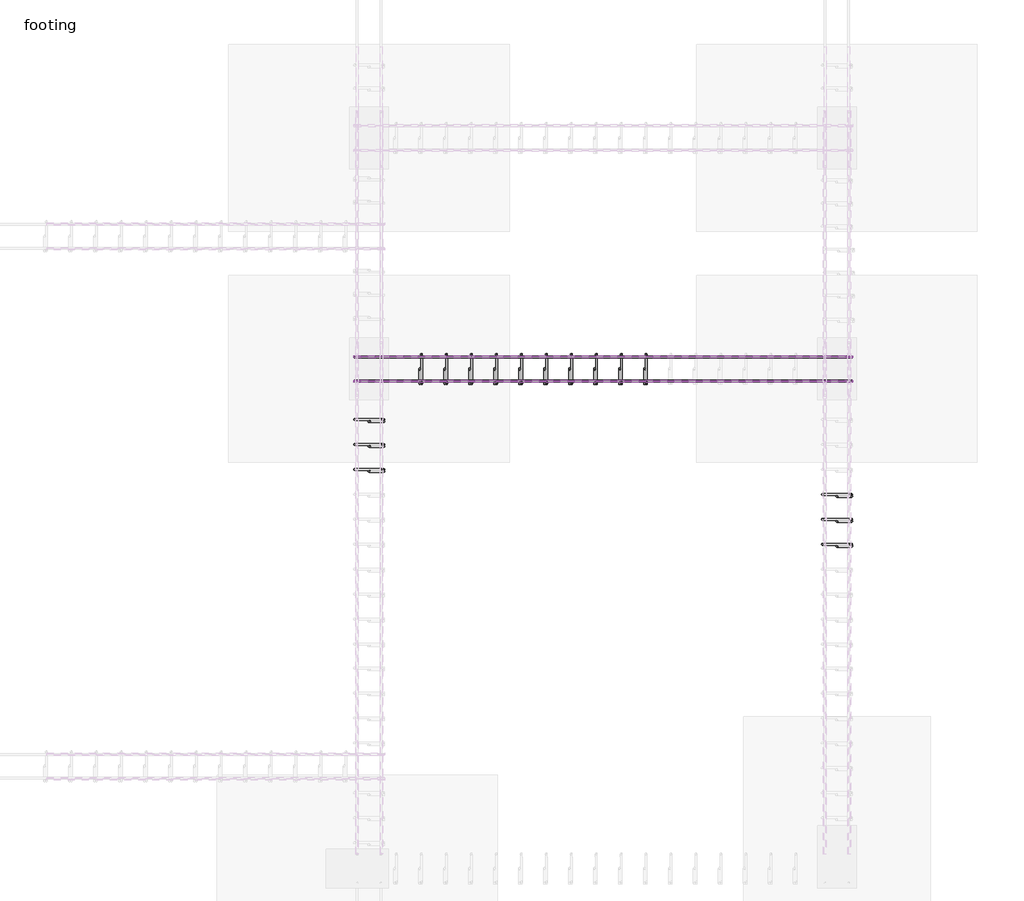
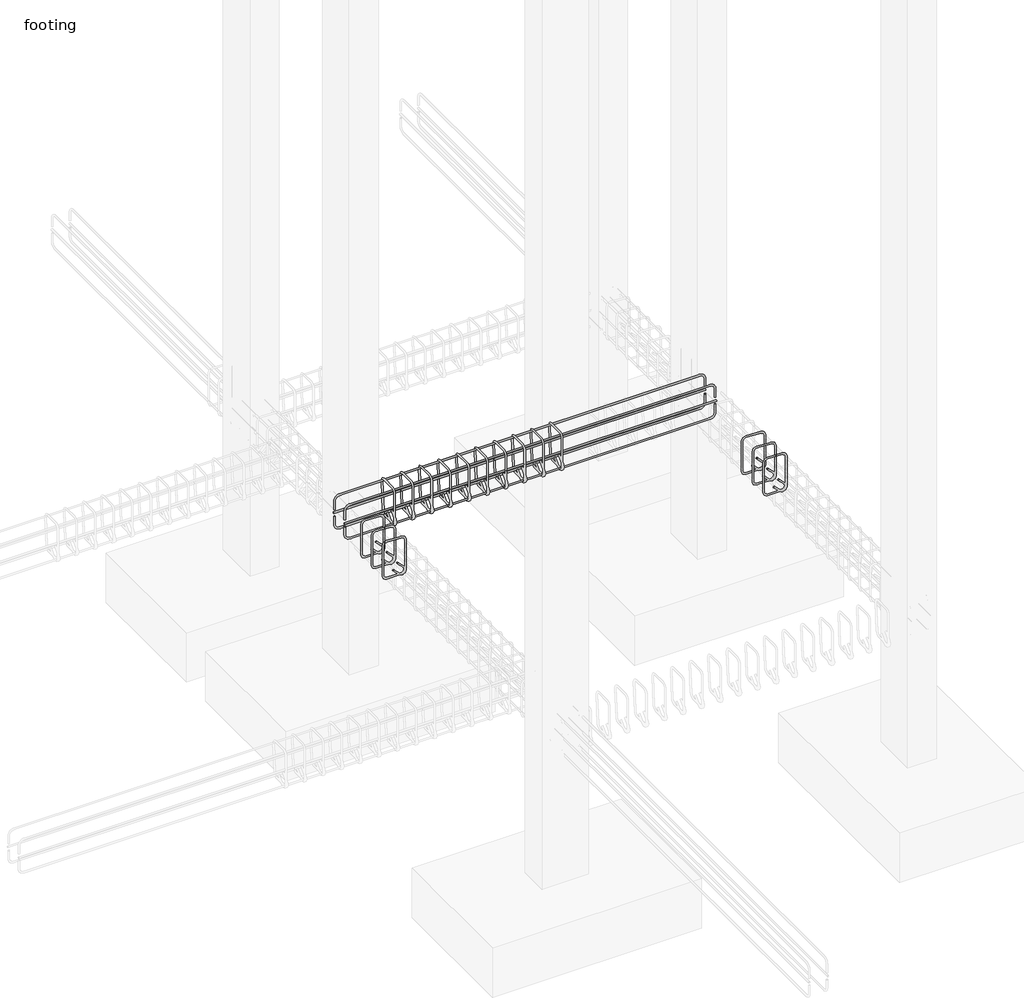
# One storey, part 13 of 21: 22 reinforcing bars.
"""IFC4 building model written with IfcOpenShell, lengths in millimetres."""

from ifc_helpers import new_model, si_unit, point, frame, origin, place, context, project, spatial, polyline, circle_curve, trimmed, segment, composite_curve, element, save
from ifc_brep_helpers import swept_disk

model = new_model("IFC4")

# Units and contexts
model_context = context("Model", 3, world=origin())
ifc_project = project(units=[si_unit("LENGTHUNIT", "METRE", prefix="MILLI")], contexts=[model_context])

# Site, building, storey
site = spatial("IfcSite", under=ifc_project)
building = spatial("IfcBuilding", under=site)
storey = spatial("IfcBuildingStorey", under=building, Name="footing", Elevation=-1524.0)

# Reinforcing bars
placement = place(None, origin())
element("IfcReinforcingBar", 1, at=placement, inside=storey, context=model_context, shape_type="SolidModel", body=[
    swept_disk(composite_curve([segment(polyline([(-4722.5521673, 6772.6372086, -236.1172592), (-4722.5521673, 6772.6372086, -312.3172592)]), True, "CONTINUOUS"), segment(trimmed(circle_curve(frame((-4767.0021673, 6772.6372086, -312.3172592), z_axis=(0.0, 1.0, -2.1166279873208456e-12), x_axis=(44.44999999999982, 0.0, 0.0)), 44.45), [point((-4722.5521673, 6772.6372086, -312.3172592))], [point((-4767.0021673, 6772.6372086, -356.7672592))], True, "CARTESIAN"), True, "CONTINUOUS"), segment(polyline([(-4767.0021673, 6772.6372086, -356.7672592), (-7917.3959173, 6772.6372086, -356.7672592)]), True, "CONTINUOUS"), segment(trimmed(circle_curve(frame((-7917.3959173, 6772.6372086, -312.3172592), z_axis=(0.0, 1.0, -2.1166279873208456e-12), x_axis=(0.0, 0.0, -44.44999999999999)), 44.45), [point((-7917.3959173, 6772.6372086, -356.7672592))], [point((-7961.8459173, 6772.6372086, -312.3172592))], True, "CARTESIAN"), True, "CONTINUOUS"), segment(polyline([(-7961.8459173, 6772.6372086, -312.3172592), (-7961.8459173, 6772.6372086, -236.1172592)]), True, "CONTINUOUS")], self_intersect=False), 6.35),
])
element("IfcReinforcingBar", 2, at=placement, inside=storey, context=model_context, shape_type="SolidModel", body=[
    swept_disk(composite_curve([segment(polyline([(-4722.5521673, 6617.9026902, -170.2827408), (-4722.5521673, 6617.9026902, -94.0827408)]), True, "CONTINUOUS"), segment(trimmed(circle_curve(frame((-4767.0021673, 6617.9026902, -94.0827408), z_axis=(0.0, -1.0, 0.0), x_axis=(44.44999999999982, 0.0, 0.0)), 44.45), [point((-4722.5521673, 6617.9026902, -94.0827408))], [point((-4767.0021673, 6617.9026902, -49.6327408))], True, "CARTESIAN"), True, "CONTINUOUS"), segment(polyline([(-4767.0021673, 6617.9026902, -49.6327408), (-7917.3959173, 6617.9026902, -49.6327408)]), True, "CONTINUOUS"), segment(trimmed(circle_curve(frame((-7917.3959173, 6617.9026902, -94.0827408), z_axis=(0.0, -1.0, 0.0), x_axis=(0.0, 0.0, 44.449999999999996)), 44.45), [point((-7917.3959173, 6617.9026902, -49.6327408))], [point((-7961.8459173, 6617.9026902, -94.0827408))], True, "CARTESIAN"), True, "CONTINUOUS"), segment(polyline([(-7961.8459173, 6617.9026902, -94.0827408), (-7961.8459173, 6617.9026902, -170.2827408)]), True, "CONTINUOUS")], self_intersect=False), 6.35),
])
element("IfcReinforcingBar", 3, at=placement, inside=storey, context=model_context, shape_type="SolidModel", body=[
    swept_disk(composite_curve([segment(polyline([(-4722.5521673, 6617.9026902, -236.1172592), (-4722.5521673, 6617.9026902, -312.3172592)]), True, "CONTINUOUS"), segment(trimmed(circle_curve(frame((-4767.0021673, 6617.9026902, -312.3172592), z_axis=(0.0, 1.0, 2.1166279873208456e-12), x_axis=(44.44999999999982, 0.0, 0.0)), 44.45), [point((-4722.5521673, 6617.9026902, -312.3172592))], [point((-4767.0021673, 6617.9026902, -356.7672592))], True, "CARTESIAN"), True, "CONTINUOUS"), segment(polyline([(-4767.0021673, 6617.9026902, -356.7672592), (-7917.3959173, 6617.9026902, -356.7672592)]), True, "CONTINUOUS"), segment(trimmed(circle_curve(frame((-7917.3959173, 6617.9026902, -312.3172592), z_axis=(0.0, 1.0, 2.1166279873208456e-12), x_axis=(0.0, 0.0, -44.44999999999999)), 44.45), [point((-7917.3959173, 6617.9026902, -356.7672592))], [point((-7961.8459173, 6617.9026902, -312.3172592))], True, "CARTESIAN"), True, "CONTINUOUS"), segment(polyline([(-7961.8459173, 6617.9026902, -312.3172592), (-7961.8459173, 6617.9026902, -236.1172592)]), True, "CONTINUOUS")], self_intersect=False), 6.35),
])
element("IfcReinforcingBar", 4, at=placement, inside=storey, context=model_context, shape_type="SolidModel", body=[
    swept_disk(composite_curve([segment(polyline([(-4722.5521673, 6772.6372086, -170.2827408), (-4722.5521673, 6772.6372086, -94.0827408)]), True, "CONTINUOUS"), segment(trimmed(circle_curve(frame((-4767.0021673, 6772.6372086, -94.0827408), z_axis=(0.0, -1.0, 0.0), x_axis=(44.44999999999982, 0.0, 0.0)), 44.45), [point((-4722.5521673, 6772.6372086, -94.0827408))], [point((-4767.0021673, 6772.6372086, -49.6327408))], True, "CARTESIAN"), True, "CONTINUOUS"), segment(polyline([(-4767.0021673, 6772.6372086, -49.6327408), (-7917.3959173, 6772.6372086, -49.6327408)]), True, "CONTINUOUS"), segment(trimmed(circle_curve(frame((-7917.3959173, 6772.6372086, -94.0827408), z_axis=(0.0, -1.0, 0.0), x_axis=(0.0, 0.0, 44.449999999999996)), 44.45), [point((-7917.3959173, 6772.6372086, -49.6327408))], [point((-7961.8459173, 6772.6372086, -94.0827408))], True, "CARTESIAN"), True, "CONTINUOUS"), segment(polyline([(-7961.8459173, 6772.6372086, -94.0827408), (-7961.8459173, 6772.6372086, -170.2827408)]), True, "CONTINUOUS")], self_intersect=False), 6.35),
])
element("IfcReinforcingBar", 5, at=placement, inside=storey, context=model_context, shape_type="SolidModel", body=[
    swept_disk(composite_curve([segment(polyline([(-4716.2021673, 6778.2168244, -203.2), (-7968.1959173, 6778.2168244, -203.2)]), True, "CONTINUOUS")], self_intersect=False), 6.35),
])
element("IfcReinforcingBar", 6, at=placement, inside=storey, context=model_context, shape_type="SolidModel", body=[
    swept_disk(composite_curve([segment(polyline([(-4716.2021673, 6612.3230744, -203.2), (-7968.1959173, 6612.3230744, -203.2)]), True, "CONTINUOUS")], self_intersect=False), 6.35),
])
element("IfcReinforcingBar", 7, at=placement, inside=storey, context=model_context, shape_type="SolidModel", body=[
    swept_disk(composite_curve([segment(polyline([(-7537.0883428, 6708.6887132, -310.8825168), (-7537.0883428, 6653.8237147, -365.7475153)]), True, "CONTINUOUS"), segment(trimmed(circle_curve(frame((-7537.0883428, 6631.3730744, -343.296875), z_axis=(-1.0, 0.0, 0.0), x_axis=(0.0, 22.450640299999577, -22.450640299999975)), 31.75), [point((-7537.0883428, 6653.8237147, -365.7475153))], [point((-7537.0883428, 6599.6230744, -343.296875))], True, "CARTESIAN"), True, "CONTINUOUS"), segment(polyline([(-7537.0883428, 6599.6230744, -343.296875), (-7537.0883428, 6599.6230744, -63.103125)]), True, "CONTINUOUS"), segment(trimmed(circle_curve(frame((-7537.0883428, 6631.3730744, -63.103125), z_axis=(-1.0, 0.0, 0.0), x_axis=(0.0, -31.75, 0.0)), 31.75), [point((-7537.0883428, 6599.6230744, -63.103125))], [point((-7537.0883428, 6631.3730744, -31.353125))], True, "CARTESIAN"), True, "CONTINUOUS"), segment(polyline([(-7537.0883428, 6631.3730744, -31.353125), (-7537.0883428, 6759.1668244, -31.353125)]), True, "CONTINUOUS"), segment(trimmed(circle_curve(frame((-7535.9159328, 6759.1668244, -63.0814712), z_axis=(-0.9993179916193466, 0.0, -0.03692629992126919), x_axis=(-1.1724100000001272, 0.0, 31.728346200000004)), 31.75), [point((-7537.0883428, 6759.1668244, -31.353125))], [point((-7535.9159328, 6790.9168244, -63.0814712))], True, "CARTESIAN"), True, "CONTINUOUS"), segment(polyline([(-7535.9159328, 6790.9168244, -63.0814712), (-7525.5607528, 6790.9168244, -343.3185288)]), True, "CONTINUOUS"), segment(trimmed(circle_curve(frame((-7525.5607528, 6759.1668244, -343.3185288), z_axis=(-0.9993179916193466, 0.0, -0.03692629992126919), x_axis=(0.0, 31.75, 0.0)), 31.75), [point((-7525.5607528, 6790.9168244, -343.3185288))], [point((-7524.3883428, 6759.1668244, -375.046875))], True, "CARTESIAN"), True, "CONTINUOUS"), segment(polyline([(-7524.3883428, 6759.1668244, -375.046875), (-7524.3883428, 6631.3730744, -375.046875)]), True, "CONTINUOUS"), segment(trimmed(circle_curve(frame((-7524.3883428, 6631.3730744, -343.296875), z_axis=(-1.0, 0.0, 0.0), x_axis=(0.0, 0.0, -31.75)), 31.75), [point((-7524.3883428, 6631.3730744, -375.046875))], [point((-7524.3883428, 6608.9224341, -320.8462347))], True, "CARTESIAN"), True, "CONTINUOUS"), segment(polyline([(-7524.3883428, 6608.9224341, -320.8462347), (-7524.3883428, 6663.7874326, -265.9812362)]), True, "CONTINUOUS")], self_intersect=False), 6.35),
])
element("IfcReinforcingBar", 8, at=placement, inside=storey, context=model_context, shape_type="SolidModel", body=[
    swept_disk(composite_curve([segment(polyline([(-7374.3883428, 6708.6887132, -310.8825168), (-7374.3883428, 6653.8237147, -365.7475153)]), True, "CONTINUOUS"), segment(trimmed(circle_curve(frame((-7374.3883428, 6631.3730744, -343.296875), z_axis=(-1.0, 0.0, 0.0), x_axis=(0.0, 22.450640299999577, -22.450640299999975)), 31.75), [point((-7374.3883428, 6653.8237147, -365.7475153))], [point((-7374.3883428, 6599.6230744, -343.296875))], True, "CARTESIAN"), True, "CONTINUOUS"), segment(polyline([(-7374.3883428, 6599.6230744, -343.296875), (-7374.3883428, 6599.6230744, -63.103125)]), True, "CONTINUOUS"), segment(trimmed(circle_curve(frame((-7374.3883428, 6631.3730744, -63.103125), z_axis=(-1.0, 0.0, 0.0), x_axis=(0.0, -31.75, 0.0)), 31.75), [point((-7374.3883428, 6599.6230744, -63.103125))], [point((-7374.3883428, 6631.3730744, -31.353125))], True, "CARTESIAN"), True, "CONTINUOUS"), segment(polyline([(-7374.3883428, 6631.3730744, -31.353125), (-7374.3883428, 6759.1668244, -31.353125)]), True, "CONTINUOUS"), segment(trimmed(circle_curve(frame((-7373.2159328, 6759.1668244, -63.0814712), z_axis=(-0.9993179916193466, 0.0, -0.03692629992126919), x_axis=(-1.1724100000001272, 0.0, 31.728346200000004)), 31.75), [point((-7374.3883428, 6759.1668244, -31.353125))], [point((-7373.2159328, 6790.9168244, -63.0814712))], True, "CARTESIAN"), True, "CONTINUOUS"), segment(polyline([(-7373.2159328, 6790.9168244, -63.0814712), (-7362.8607528, 6790.9168244, -343.3185288)]), True, "CONTINUOUS"), segment(trimmed(circle_curve(frame((-7362.8607528, 6759.1668244, -343.3185288), z_axis=(-0.9993179916193466, 0.0, -0.03692629992126919), x_axis=(0.0, 31.75, 0.0)), 31.75), [point((-7362.8607528, 6790.9168244, -343.3185288))], [point((-7361.6883428, 6759.1668244, -375.046875))], True, "CARTESIAN"), True, "CONTINUOUS"), segment(polyline([(-7361.6883428, 6759.1668244, -375.046875), (-7361.6883428, 6631.3730744, -375.046875)]), True, "CONTINUOUS"), segment(trimmed(circle_curve(frame((-7361.6883428, 6631.3730744, -343.296875), z_axis=(-1.0, 0.0, 0.0), x_axis=(0.0, 0.0, -31.75)), 31.75), [point((-7361.6883428, 6631.3730744, -375.046875))], [point((-7361.6883428, 6608.9224341, -320.8462347))], True, "CARTESIAN"), True, "CONTINUOUS"), segment(polyline([(-7361.6883428, 6608.9224341, -320.8462347), (-7361.6883428, 6663.7874326, -265.9812362)]), True, "CONTINUOUS")], self_intersect=False), 6.35),
])
element("IfcReinforcingBar", 9, at=placement, inside=storey, context=model_context, shape_type="SolidModel", body=[
    swept_disk(composite_curve([segment(polyline([(-7211.6883428, 6708.6887132, -310.8825168), (-7211.6883428, 6653.8237147, -365.7475153)]), True, "CONTINUOUS"), segment(trimmed(circle_curve(frame((-7211.6883428, 6631.3730744, -343.296875), z_axis=(-1.0, 0.0, 0.0), x_axis=(0.0, 22.450640299999577, -22.450640299999975)), 31.75), [point((-7211.6883428, 6653.8237147, -365.7475153))], [point((-7211.6883428, 6599.6230744, -343.296875))], True, "CARTESIAN"), True, "CONTINUOUS"), segment(polyline([(-7211.6883428, 6599.6230744, -343.296875), (-7211.6883428, 6599.6230744, -63.103125)]), True, "CONTINUOUS"), segment(trimmed(circle_curve(frame((-7211.6883428, 6631.3730744, -63.103125), z_axis=(-1.0, 0.0, 0.0), x_axis=(0.0, -31.75, 0.0)), 31.75), [point((-7211.6883428, 6599.6230744, -63.103125))], [point((-7211.6883428, 6631.3730744, -31.353125))], True, "CARTESIAN"), True, "CONTINUOUS"), segment(polyline([(-7211.6883428, 6631.3730744, -31.353125), (-7211.6883428, 6759.1668244, -31.353125)]), True, "CONTINUOUS"), segment(trimmed(circle_curve(frame((-7210.5159328, 6759.1668244, -63.0814712), z_axis=(-0.9993179916193466, 0.0, -0.03692629992126919), x_axis=(-1.1724100000001272, 0.0, 31.728346200000004)), 31.75), [point((-7211.6883428, 6759.1668244, -31.353125))], [point((-7210.5159328, 6790.9168244, -63.0814712))], True, "CARTESIAN"), True, "CONTINUOUS"), segment(polyline([(-7210.5159328, 6790.9168244, -63.0814712), (-7200.1607528, 6790.9168244, -343.3185288)]), True, "CONTINUOUS"), segment(trimmed(circle_curve(frame((-7200.1607528, 6759.1668244, -343.3185288), z_axis=(-0.9993179916193466, 0.0, -0.03692629992126919), x_axis=(0.0, 31.75, 0.0)), 31.75), [point((-7200.1607528, 6790.9168244, -343.3185288))], [point((-7198.9883428, 6759.1668244, -375.046875))], True, "CARTESIAN"), True, "CONTINUOUS"), segment(polyline([(-7198.9883428, 6759.1668244, -375.046875), (-7198.9883428, 6631.3730744, -375.046875)]), True, "CONTINUOUS"), segment(trimmed(circle_curve(frame((-7198.9883428, 6631.3730744, -343.296875), z_axis=(-1.0, 0.0, 0.0), x_axis=(0.0, 0.0, -31.75)), 31.75), [point((-7198.9883428, 6631.3730744, -375.046875))], [point((-7198.9883428, 6608.9224341, -320.8462347))], True, "CARTESIAN"), True, "CONTINUOUS"), segment(polyline([(-7198.9883428, 6608.9224341, -320.8462347), (-7198.9883428, 6663.7874326, -265.9812362)]), True, "CONTINUOUS")], self_intersect=False), 6.35),
])
element("IfcReinforcingBar", 10, at=placement, inside=storey, context=model_context, shape_type="SolidModel", body=[
    swept_disk(composite_curve([segment(polyline([(-7048.9883428, 6708.6887132, -310.8825168), (-7048.9883428, 6653.8237147, -365.7475153)]), True, "CONTINUOUS"), segment(trimmed(circle_curve(frame((-7048.9883428, 6631.3730744, -343.296875), z_axis=(-1.0, 0.0, 0.0), x_axis=(0.0, 22.450640299999577, -22.450640299999975)), 31.75), [point((-7048.9883428, 6653.8237147, -365.7475153))], [point((-7048.9883428, 6599.6230744, -343.296875))], True, "CARTESIAN"), True, "CONTINUOUS"), segment(polyline([(-7048.9883428, 6599.6230744, -343.296875), (-7048.9883428, 6599.6230744, -63.103125)]), True, "CONTINUOUS"), segment(trimmed(circle_curve(frame((-7048.9883428, 6631.3730744, -63.103125), z_axis=(-1.0, 0.0, 0.0), x_axis=(0.0, -31.75, 0.0)), 31.75), [point((-7048.9883428, 6599.6230744, -63.103125))], [point((-7048.9883428, 6631.3730744, -31.353125))], True, "CARTESIAN"), True, "CONTINUOUS"), segment(polyline([(-7048.9883428, 6631.3730744, -31.353125), (-7048.9883428, 6759.1668244, -31.353125)]), True, "CONTINUOUS"), segment(trimmed(circle_curve(frame((-7047.8159328, 6759.1668244, -63.0814712), z_axis=(-0.9993179916193466, 0.0, -0.03692629992126919), x_axis=(-1.1724100000001272, 0.0, 31.728346200000004)), 31.75), [point((-7048.9883428, 6759.1668244, -31.353125))], [point((-7047.8159328, 6790.9168244, -63.0814712))], True, "CARTESIAN"), True, "CONTINUOUS"), segment(polyline([(-7047.8159328, 6790.9168244, -63.0814712), (-7037.4607528, 6790.9168244, -343.3185288)]), True, "CONTINUOUS"), segment(trimmed(circle_curve(frame((-7037.4607528, 6759.1668244, -343.3185288), z_axis=(-0.9993179916193466, 0.0, -0.03692629992126919), x_axis=(0.0, 31.75, 0.0)), 31.75), [point((-7037.4607528, 6790.9168244, -343.3185288))], [point((-7036.2883428, 6759.1668244, -375.046875))], True, "CARTESIAN"), True, "CONTINUOUS"), segment(polyline([(-7036.2883428, 6759.1668244, -375.046875), (-7036.2883428, 6631.3730744, -375.046875)]), True, "CONTINUOUS"), segment(trimmed(circle_curve(frame((-7036.2883428, 6631.3730744, -343.296875), z_axis=(-1.0, 0.0, 0.0), x_axis=(0.0, 0.0, -31.75)), 31.75), [point((-7036.2883428, 6631.3730744, -375.046875))], [point((-7036.2883428, 6608.9224341, -320.8462347))], True, "CARTESIAN"), True, "CONTINUOUS"), segment(polyline([(-7036.2883428, 6608.9224341, -320.8462347), (-7036.2883428, 6663.7874326, -265.9812362)]), True, "CONTINUOUS")], self_intersect=False), 6.35),
])
element("IfcReinforcingBar", 11, at=placement, inside=storey, context=model_context, shape_type="SolidModel", body=[
    swept_disk(composite_curve([segment(polyline([(-6886.2883428, 6708.6887132, -310.8825168), (-6886.2883428, 6653.8237147, -365.7475153)]), True, "CONTINUOUS"), segment(trimmed(circle_curve(frame((-6886.2883428, 6631.3730744, -343.296875), z_axis=(-1.0, 0.0, 0.0), x_axis=(0.0, 22.450640299999577, -22.450640299999975)), 31.75), [point((-6886.2883428, 6653.8237147, -365.7475153))], [point((-6886.2883428, 6599.6230744, -343.296875))], True, "CARTESIAN"), True, "CONTINUOUS"), segment(polyline([(-6886.2883428, 6599.6230744, -343.296875), (-6886.2883428, 6599.6230744, -63.103125)]), True, "CONTINUOUS"), segment(trimmed(circle_curve(frame((-6886.2883428, 6631.3730744, -63.103125), z_axis=(-1.0, 0.0, 0.0), x_axis=(0.0, -31.75, 0.0)), 31.75), [point((-6886.2883428, 6599.6230744, -63.103125))], [point((-6886.2883428, 6631.3730744, -31.353125))], True, "CARTESIAN"), True, "CONTINUOUS"), segment(polyline([(-6886.2883428, 6631.3730744, -31.353125), (-6886.2883428, 6759.1668244, -31.353125)]), True, "CONTINUOUS"), segment(trimmed(circle_curve(frame((-6885.1159328, 6759.1668244, -63.0814712), z_axis=(-0.9993179916193466, 0.0, -0.03692629992126919), x_axis=(-1.1724099999992177, 0.0, 31.728346200000004)), 31.75), [point((-6886.2883428, 6759.1668244, -31.353125))], [point((-6885.1159328, 6790.9168244, -63.0814712))], True, "CARTESIAN"), True, "CONTINUOUS"), segment(polyline([(-6885.1159328, 6790.9168244, -63.0814712), (-6874.7607528, 6790.9168244, -343.3185288)]), True, "CONTINUOUS"), segment(trimmed(circle_curve(frame((-6874.7607528, 6759.1668244, -343.3185288), z_axis=(-0.9993179916193466, 0.0, -0.03692629992126919), x_axis=(0.0, 31.75, 0.0)), 31.75), [point((-6874.7607528, 6790.9168244, -343.3185288))], [point((-6873.5883428, 6759.1668244, -375.046875))], True, "CARTESIAN"), True, "CONTINUOUS"), segment(polyline([(-6873.5883428, 6759.1668244, -375.046875), (-6873.5883428, 6631.3730744, -375.046875)]), True, "CONTINUOUS"), segment(trimmed(circle_curve(frame((-6873.5883428, 6631.3730744, -343.296875), z_axis=(-1.0, 0.0, 0.0), x_axis=(0.0, 0.0, -31.75)), 31.75), [point((-6873.5883428, 6631.3730744, -375.046875))], [point((-6873.5883428, 6608.9224341, -320.8462347))], True, "CARTESIAN"), True, "CONTINUOUS"), segment(polyline([(-6873.5883428, 6608.9224341, -320.8462347), (-6873.5883428, 6663.7874326, -265.9812362)]), True, "CONTINUOUS")], self_intersect=False), 6.35),
])
element("IfcReinforcingBar", 12, at=placement, inside=storey, context=model_context, shape_type="SolidModel", body=[
    swept_disk(composite_curve([segment(polyline([(-6723.5883428, 6708.6887132, -310.8825168), (-6723.5883428, 6653.8237147, -365.7475153)]), True, "CONTINUOUS"), segment(trimmed(circle_curve(frame((-6723.5883428, 6631.3730744, -343.296875), z_axis=(-1.0, 0.0, 0.0), x_axis=(0.0, 22.450640299999577, -22.450640299999975)), 31.75), [point((-6723.5883428, 6653.8237147, -365.7475153))], [point((-6723.5883428, 6599.6230744, -343.296875))], True, "CARTESIAN"), True, "CONTINUOUS"), segment(polyline([(-6723.5883428, 6599.6230744, -343.296875), (-6723.5883428, 6599.6230744, -63.103125)]), True, "CONTINUOUS"), segment(trimmed(circle_curve(frame((-6723.5883428, 6631.3730744, -63.103125), z_axis=(-1.0, 0.0, 0.0), x_axis=(0.0, -31.75, 0.0)), 31.75), [point((-6723.5883428, 6599.6230744, -63.103125))], [point((-6723.5883428, 6631.3730744, -31.353125))], True, "CARTESIAN"), True, "CONTINUOUS"), segment(polyline([(-6723.5883428, 6631.3730744, -31.353125), (-6723.5883428, 6759.1668244, -31.353125)]), True, "CONTINUOUS"), segment(trimmed(circle_curve(frame((-6722.4159328, 6759.1668244, -63.0814712), z_axis=(-0.9993179916193466, 0.0, -0.03692629992126919), x_axis=(-1.1724100000001272, 0.0, 31.728346200000004)), 31.75), [point((-6723.5883428, 6759.1668244, -31.353125))], [point((-6722.4159328, 6790.9168244, -63.0814712))], True, "CARTESIAN"), True, "CONTINUOUS"), segment(polyline([(-6722.4159328, 6790.9168244, -63.0814712), (-6712.0607528, 6790.9168244, -343.3185288)]), True, "CONTINUOUS"), segment(trimmed(circle_curve(frame((-6712.0607528, 6759.1668244, -343.3185288), z_axis=(-0.9993179916193466, 0.0, -0.03692629992126919), x_axis=(0.0, 31.75, 0.0)), 31.75), [point((-6712.0607528, 6790.9168244, -343.3185288))], [point((-6710.8883428, 6759.1668244, -375.046875))], True, "CARTESIAN"), True, "CONTINUOUS"), segment(polyline([(-6710.8883428, 6759.1668244, -375.046875), (-6710.8883428, 6631.3730744, -375.046875)]), True, "CONTINUOUS"), segment(trimmed(circle_curve(frame((-6710.8883428, 6631.3730744, -343.296875), z_axis=(-1.0, 0.0, 0.0), x_axis=(0.0, 0.0, -31.75)), 31.75), [point((-6710.8883428, 6631.3730744, -375.046875))], [point((-6710.8883428, 6608.9224341, -320.8462347))], True, "CARTESIAN"), True, "CONTINUOUS"), segment(polyline([(-6710.8883428, 6608.9224341, -320.8462347), (-6710.8883428, 6663.7874326, -265.9812362)]), True, "CONTINUOUS")], self_intersect=False), 6.35),
])
element("IfcReinforcingBar", 13, at=placement, inside=storey, context=model_context, shape_type="SolidModel", body=[
    swept_disk(composite_curve([segment(polyline([(-6560.8883428, 6708.6887132, -310.8825168), (-6560.8883428, 6653.8237147, -365.7475153)]), True, "CONTINUOUS"), segment(trimmed(circle_curve(frame((-6560.8883428, 6631.3730744, -343.296875), z_axis=(-1.0, 0.0, 0.0), x_axis=(0.0, 22.450640299999577, -22.450640299999975)), 31.75), [point((-6560.8883428, 6653.8237147, -365.7475153))], [point((-6560.8883428, 6599.6230744, -343.296875))], True, "CARTESIAN"), True, "CONTINUOUS"), segment(polyline([(-6560.8883428, 6599.6230744, -343.296875), (-6560.8883428, 6599.6230744, -63.103125)]), True, "CONTINUOUS"), segment(trimmed(circle_curve(frame((-6560.8883428, 6631.3730744, -63.103125), z_axis=(-1.0, 0.0, 0.0), x_axis=(0.0, -31.75, 0.0)), 31.75), [point((-6560.8883428, 6599.6230744, -63.103125))], [point((-6560.8883428, 6631.3730744, -31.353125))], True, "CARTESIAN"), True, "CONTINUOUS"), segment(polyline([(-6560.8883428, 6631.3730744, -31.353125), (-6560.8883428, 6759.1668244, -31.353125)]), True, "CONTINUOUS"), segment(trimmed(circle_curve(frame((-6559.7159328, 6759.1668244, -63.0814712), z_axis=(-0.9993179916193466, 0.0, -0.03692629992126919), x_axis=(-1.1724100000001272, 0.0, 31.728346200000004)), 31.75), [point((-6560.8883428, 6759.1668244, -31.353125))], [point((-6559.7159328, 6790.9168244, -63.0814712))], True, "CARTESIAN"), True, "CONTINUOUS"), segment(polyline([(-6559.7159328, 6790.9168244, -63.0814712), (-6549.3607528, 6790.9168244, -343.3185288)]), True, "CONTINUOUS"), segment(trimmed(circle_curve(frame((-6549.3607528, 6759.1668244, -343.3185288), z_axis=(-0.9993179916193466, 0.0, -0.03692629992126919), x_axis=(0.0, 31.75, 0.0)), 31.75), [point((-6549.3607528, 6790.9168244, -343.3185288))], [point((-6548.1883428, 6759.1668244, -375.046875))], True, "CARTESIAN"), True, "CONTINUOUS"), segment(polyline([(-6548.1883428, 6759.1668244, -375.046875), (-6548.1883428, 6631.3730744, -375.046875)]), True, "CONTINUOUS"), segment(trimmed(circle_curve(frame((-6548.1883428, 6631.3730744, -343.296875), z_axis=(-1.0, 0.0, 0.0), x_axis=(0.0, 0.0, -31.75)), 31.75), [point((-6548.1883428, 6631.3730744, -375.046875))], [point((-6548.1883428, 6608.9224341, -320.8462347))], True, "CARTESIAN"), True, "CONTINUOUS"), segment(polyline([(-6548.1883428, 6608.9224341, -320.8462347), (-6548.1883428, 6663.7874326, -265.9812362)]), True, "CONTINUOUS")], self_intersect=False), 6.35),
])
element("IfcReinforcingBar", 14, at=placement, inside=storey, context=model_context, shape_type="SolidModel", body=[
    swept_disk(composite_curve([segment(polyline([(-6398.1883428, 6708.6887132, -310.8825168), (-6398.1883428, 6653.8237147, -365.7475153)]), True, "CONTINUOUS"), segment(trimmed(circle_curve(frame((-6398.1883428, 6631.3730744, -343.296875), z_axis=(-1.0, 0.0, 0.0), x_axis=(0.0, 22.450640299999577, -22.450640299999975)), 31.75), [point((-6398.1883428, 6653.8237147, -365.7475153))], [point((-6398.1883428, 6599.6230744, -343.296875))], True, "CARTESIAN"), True, "CONTINUOUS"), segment(polyline([(-6398.1883428, 6599.6230744, -343.296875), (-6398.1883428, 6599.6230744, -63.103125)]), True, "CONTINUOUS"), segment(trimmed(circle_curve(frame((-6398.1883428, 6631.3730744, -63.103125), z_axis=(-1.0, 0.0, 0.0), x_axis=(0.0, -31.75, 0.0)), 31.75), [point((-6398.1883428, 6599.6230744, -63.103125))], [point((-6398.1883428, 6631.3730744, -31.353125))], True, "CARTESIAN"), True, "CONTINUOUS"), segment(polyline([(-6398.1883428, 6631.3730744, -31.353125), (-6398.1883428, 6759.1668244, -31.353125)]), True, "CONTINUOUS"), segment(trimmed(circle_curve(frame((-6397.0159328, 6759.1668244, -63.0814712), z_axis=(-0.9993179916193466, 0.0, -0.03692629992126919), x_axis=(-1.1724100000001272, 0.0, 31.728346200000004)), 31.75), [point((-6398.1883428, 6759.1668244, -31.353125))], [point((-6397.0159328, 6790.9168244, -63.0814712))], True, "CARTESIAN"), True, "CONTINUOUS"), segment(polyline([(-6397.0159328, 6790.9168244, -63.0814712), (-6386.6607528, 6790.9168244, -343.3185288)]), True, "CONTINUOUS"), segment(trimmed(circle_curve(frame((-6386.6607528, 6759.1668244, -343.3185288), z_axis=(-0.9993179916193466, 0.0, -0.03692629992126919), x_axis=(0.0, 31.75, 0.0)), 31.75), [point((-6386.6607528, 6790.9168244, -343.3185288))], [point((-6385.4883428, 6759.1668244, -375.046875))], True, "CARTESIAN"), True, "CONTINUOUS"), segment(polyline([(-6385.4883428, 6759.1668244, -375.046875), (-6385.4883428, 6631.3730744, -375.046875)]), True, "CONTINUOUS"), segment(trimmed(circle_curve(frame((-6385.4883428, 6631.3730744, -343.296875), z_axis=(-1.0, 0.0, 0.0), x_axis=(0.0, 0.0, -31.75)), 31.75), [point((-6385.4883428, 6631.3730744, -375.046875))], [point((-6385.4883428, 6608.9224341, -320.8462347))], True, "CARTESIAN"), True, "CONTINUOUS"), segment(polyline([(-6385.4883428, 6608.9224341, -320.8462347), (-6385.4883428, 6663.7874326, -265.9812362)]), True, "CONTINUOUS")], self_intersect=False), 6.35),
])
element("IfcReinforcingBar", 15, at=placement, inside=storey, context=model_context, shape_type="SolidModel", body=[
    swept_disk(composite_curve([segment(polyline([(-6235.4883428, 6708.6887132, -310.8825168), (-6235.4883428, 6653.8237147, -365.7475153)]), True, "CONTINUOUS"), segment(trimmed(circle_curve(frame((-6235.4883428, 6631.3730744, -343.296875), z_axis=(-1.0, 0.0, 0.0), x_axis=(0.0, 22.450640299999577, -22.450640299999975)), 31.75), [point((-6235.4883428, 6653.8237147, -365.7475153))], [point((-6235.4883428, 6599.6230744, -343.296875))], True, "CARTESIAN"), True, "CONTINUOUS"), segment(polyline([(-6235.4883428, 6599.6230744, -343.296875), (-6235.4883428, 6599.6230744, -63.103125)]), True, "CONTINUOUS"), segment(trimmed(circle_curve(frame((-6235.4883428, 6631.3730744, -63.103125), z_axis=(-1.0, 0.0, 0.0), x_axis=(0.0, -31.75, 0.0)), 31.75), [point((-6235.4883428, 6599.6230744, -63.103125))], [point((-6235.4883428, 6631.3730744, -31.353125))], True, "CARTESIAN"), True, "CONTINUOUS"), segment(polyline([(-6235.4883428, 6631.3730744, -31.353125), (-6235.4883428, 6759.1668244, -31.353125)]), True, "CONTINUOUS"), segment(trimmed(circle_curve(frame((-6234.3159328, 6759.1668244, -63.0814712), z_axis=(-0.9993179916193466, 0.0, -0.03692629992126919), x_axis=(-1.1724100000001272, 0.0, 31.728346200000004)), 31.75), [point((-6235.4883428, 6759.1668244, -31.353125))], [point((-6234.3159328, 6790.9168244, -63.0814712))], True, "CARTESIAN"), True, "CONTINUOUS"), segment(polyline([(-6234.3159328, 6790.9168244, -63.0814712), (-6223.9607528, 6790.9168244, -343.3185288)]), True, "CONTINUOUS"), segment(trimmed(circle_curve(frame((-6223.9607528, 6759.1668244, -343.3185288), z_axis=(-0.9993179916193466, 0.0, -0.03692629992126919), x_axis=(0.0, 31.75, 0.0)), 31.75), [point((-6223.9607528, 6790.9168244, -343.3185288))], [point((-6222.7883428, 6759.1668244, -375.046875))], True, "CARTESIAN"), True, "CONTINUOUS"), segment(polyline([(-6222.7883428, 6759.1668244, -375.046875), (-6222.7883428, 6631.3730744, -375.046875)]), True, "CONTINUOUS"), segment(trimmed(circle_curve(frame((-6222.7883428, 6631.3730744, -343.296875), z_axis=(-1.0, 0.0, 0.0), x_axis=(0.0, 0.0, -31.75)), 31.75), [point((-6222.7883428, 6631.3730744, -375.046875))], [point((-6222.7883428, 6608.9224341, -320.8462347))], True, "CARTESIAN"), True, "CONTINUOUS"), segment(polyline([(-6222.7883428, 6608.9224341, -320.8462347), (-6222.7883428, 6663.7874326, -265.9812362)]), True, "CONTINUOUS")], self_intersect=False), 6.35),
])
element("IfcReinforcingBar", 16, at=placement, inside=storey, context=model_context, shape_type="SolidModel", body=[
    swept_disk(composite_curve([segment(polyline([(-6072.7883428, 6708.6887132, -310.8825168), (-6072.7883428, 6653.8237147, -365.7475153)]), True, "CONTINUOUS"), segment(trimmed(circle_curve(frame((-6072.7883428, 6631.3730744, -343.296875), z_axis=(-1.0, 0.0, 0.0), x_axis=(0.0, 22.450640299999577, -22.450640299999975)), 31.75), [point((-6072.7883428, 6653.8237147, -365.7475153))], [point((-6072.7883428, 6599.6230744, -343.296875))], True, "CARTESIAN"), True, "CONTINUOUS"), segment(polyline([(-6072.7883428, 6599.6230744, -343.296875), (-6072.7883428, 6599.6230744, -63.103125)]), True, "CONTINUOUS"), segment(trimmed(circle_curve(frame((-6072.7883428, 6631.3730744, -63.103125), z_axis=(-1.0, 0.0, 0.0), x_axis=(0.0, -31.75, 0.0)), 31.75), [point((-6072.7883428, 6599.6230744, -63.103125))], [point((-6072.7883428, 6631.3730744, -31.353125))], True, "CARTESIAN"), True, "CONTINUOUS"), segment(polyline([(-6072.7883428, 6631.3730744, -31.353125), (-6072.7883428, 6759.1668244, -31.353125)]), True, "CONTINUOUS"), segment(trimmed(circle_curve(frame((-6071.6159328, 6759.1668244, -63.0814712), z_axis=(-0.9993179916193466, 0.0, -0.03692629992126919), x_axis=(-1.1724099999992177, 0.0, 31.728346200000004)), 31.75), [point((-6072.7883428, 6759.1668244, -31.353125))], [point((-6071.6159328, 6790.9168244, -63.0814712))], True, "CARTESIAN"), True, "CONTINUOUS"), segment(polyline([(-6071.6159328, 6790.9168244, -63.0814712), (-6061.2607528, 6790.9168244, -343.3185288)]), True, "CONTINUOUS"), segment(trimmed(circle_curve(frame((-6061.2607528, 6759.1668244, -343.3185288), z_axis=(-0.9993179916193466, 0.0, -0.03692629992126919), x_axis=(0.0, 31.75, 0.0)), 31.75), [point((-6061.2607528, 6790.9168244, -343.3185288))], [point((-6060.0883428, 6759.1668244, -375.046875))], True, "CARTESIAN"), True, "CONTINUOUS"), segment(polyline([(-6060.0883428, 6759.1668244, -375.046875), (-6060.0883428, 6631.3730744, -375.046875)]), True, "CONTINUOUS"), segment(trimmed(circle_curve(frame((-6060.0883428, 6631.3730744, -343.296875), z_axis=(-1.0, 0.0, 0.0), x_axis=(0.0, 0.0, -31.75)), 31.75), [point((-6060.0883428, 6631.3730744, -375.046875))], [point((-6060.0883428, 6608.9224341, -320.8462347))], True, "CARTESIAN"), True, "CONTINUOUS"), segment(polyline([(-6060.0883428, 6608.9224341, -320.8462347), (-6060.0883428, 6663.7874326, -265.9812362)]), True, "CONTINUOUS")], self_intersect=False), 6.35),
])
element("IfcReinforcingBar", 17, at=placement, inside=storey, context=model_context, shape_type="SolidModel", body=[
    swept_disk(composite_curve([segment(polyline([(-7834.7165254, 6040.4456073, -265.9812362), (-7779.851527, 6040.4456073, -320.8462347)]), True, "CONTINUOUS"), segment(trimmed(circle_curve(frame((-7802.3021673, 6040.4456073, -343.296875), z_axis=(0.0, 1.0, 0.0), x_axis=(22.450640300000487, 0.0, 22.450640299999975)), 31.75), [point((-7779.851527, 6040.4456073, -320.8462347))], [point((-7802.3021673, 6040.4456073, -375.046875))], True, "CARTESIAN"), True, "CONTINUOUS"), segment(polyline([(-7802.3021673, 6040.4456073, -375.046875), (-7930.0959173, 6040.4456073, -375.046875)]), True, "CONTINUOUS"), segment(trimmed(circle_curve(frame((-7930.0959173, 6040.4456073, -343.296875), z_axis=(0.0, 1.0, 0.0), x_axis=(0.0, 0.0, -31.75)), 31.75), [point((-7930.0959173, 6040.4456073, -375.046875))], [point((-7961.8459173, 6040.4456073, -343.296875))], True, "CARTESIAN"), True, "CONTINUOUS"), segment(polyline([(-7961.8459173, 6040.4456073, -343.296875), (-7961.8459173, 6040.4456073, -63.103125)]), True, "CONTINUOUS"), segment(trimmed(circle_curve(frame((-7930.165658, 6038.3423536, -63.103125), z_axis=(0.0662442117686417, 0.9978034397651431, 0.0), x_axis=(-31.680259300000216, 2.1032537000000957, 0.0)), 31.75), [point((-7961.8459173, 6040.4456073, -63.103125))], [point((-7930.165658, 6038.3423536, -31.353125))], True, "CARTESIAN"), True, "CONTINUOUS"), segment(polyline([(-7930.165658, 6038.3423536, -31.353125), (-7802.2324265, 6029.848861, -31.353125)]), True, "CONTINUOUS"), segment(trimmed(circle_curve(frame((-7802.2324265, 6029.848861, -63.103125), z_axis=(0.06624421176864169, 0.997803439765143, 0.0), x_axis=(0.0, 0.0, 31.75)), 31.75), [point((-7802.2324265, 6029.848861, -31.353125))], [point((-7770.5521673, 6027.7456073, -63.103125))], True, "CARTESIAN"), True, "CONTINUOUS"), segment(polyline([(-7770.5521673, 6027.7456073, -63.103125), (-7770.5521673, 6027.7456073, -343.296875)]), True, "CONTINUOUS"), segment(trimmed(circle_curve(frame((-7802.3021673, 6027.7456073, -343.296875), z_axis=(0.0, 1.0, 0.0), x_axis=(31.75, 0.0, 0.0)), 31.75), [point((-7770.5521673, 6027.7456073, -343.296875))], [point((-7824.7528076, 6027.7456073, -365.7475153))], True, "CARTESIAN"), True, "CONTINUOUS"), segment(polyline([(-7824.7528076, 6027.7456073, -365.7475153), (-7879.617806, 6027.7456073, -310.8825168)]), True, "CONTINUOUS")], self_intersect=False), 6.35),
])
element("IfcReinforcingBar", 18, at=placement, inside=storey, context=model_context, shape_type="SolidModel", body=[
    swept_disk(composite_curve([segment(polyline([(-7834.7165254, 6203.1456073, -265.9812362), (-7779.851527, 6203.1456073, -320.8462347)]), True, "CONTINUOUS"), segment(trimmed(circle_curve(frame((-7802.3021673, 6203.1456073, -343.296875), z_axis=(0.0, 1.0, 0.0), x_axis=(22.450640300000487, 0.0, 22.450640299999975)), 31.75), [point((-7779.851527, 6203.1456073, -320.8462347))], [point((-7802.3021673, 6203.1456073, -375.046875))], True, "CARTESIAN"), True, "CONTINUOUS"), segment(polyline([(-7802.3021673, 6203.1456073, -375.046875), (-7930.0959173, 6203.1456073, -375.046875)]), True, "CONTINUOUS"), segment(trimmed(circle_curve(frame((-7930.0959173, 6203.1456073, -343.296875), z_axis=(0.0, 1.0, 0.0), x_axis=(0.0, 0.0, -31.75)), 31.75), [point((-7930.0959173, 6203.1456073, -375.046875))], [point((-7961.8459173, 6203.1456073, -343.296875))], True, "CARTESIAN"), True, "CONTINUOUS"), segment(polyline([(-7961.8459173, 6203.1456073, -343.296875), (-7961.8459173, 6203.1456073, -63.103125)]), True, "CONTINUOUS"), segment(trimmed(circle_curve(frame((-7930.165658, 6201.0423536, -63.103125), z_axis=(0.0662442117686417, 0.9978034397651431, 0.0), x_axis=(-31.680259300000216, 2.1032537000000957, 0.0)), 31.75), [point((-7961.8459173, 6203.1456073, -63.103125))], [point((-7930.165658, 6201.0423536, -31.353125))], True, "CARTESIAN"), True, "CONTINUOUS"), segment(polyline([(-7930.165658, 6201.0423536, -31.353125), (-7802.2324265, 6192.548861, -31.353125)]), True, "CONTINUOUS"), segment(trimmed(circle_curve(frame((-7802.2324265, 6192.548861, -63.103125), z_axis=(0.06624421176864169, 0.997803439765143, 0.0), x_axis=(0.0, 0.0, 31.75)), 31.75), [point((-7802.2324265, 6192.548861, -31.353125))], [point((-7770.5521673, 6190.4456073, -63.103125))], True, "CARTESIAN"), True, "CONTINUOUS"), segment(polyline([(-7770.5521673, 6190.4456073, -63.103125), (-7770.5521673, 6190.4456073, -343.296875)]), True, "CONTINUOUS"), segment(trimmed(circle_curve(frame((-7802.3021673, 6190.4456073, -343.296875), z_axis=(0.0, 1.0, 0.0), x_axis=(31.75, 0.0, 0.0)), 31.75), [point((-7770.5521673, 6190.4456073, -343.296875))], [point((-7824.7528076, 6190.4456073, -365.7475153))], True, "CARTESIAN"), True, "CONTINUOUS"), segment(polyline([(-7824.7528076, 6190.4456073, -365.7475153), (-7879.617806, 6190.4456073, -310.8825168)]), True, "CONTINUOUS")], self_intersect=False), 6.35),
])
element("IfcReinforcingBar", 19, at=placement, inside=storey, context=model_context, shape_type="SolidModel", body=[
    swept_disk(composite_curve([segment(polyline([(-7834.7165254, 6365.8456073, -265.9812362), (-7779.851527, 6365.8456073, -320.8462347)]), True, "CONTINUOUS"), segment(trimmed(circle_curve(frame((-7802.3021673, 6365.8456073, -343.296875), z_axis=(0.0, 1.0, 0.0), x_axis=(22.450640300000487, 0.0, 22.450640299999975)), 31.75), [point((-7779.851527, 6365.8456073, -320.8462347))], [point((-7802.3021673, 6365.8456073, -375.046875))], True, "CARTESIAN"), True, "CONTINUOUS"), segment(polyline([(-7802.3021673, 6365.8456073, -375.046875), (-7930.0959173, 6365.8456073, -375.046875)]), True, "CONTINUOUS"), segment(trimmed(circle_curve(frame((-7930.0959173, 6365.8456073, -343.296875), z_axis=(0.0, 1.0, 0.0), x_axis=(0.0, 0.0, -31.75)), 31.75), [point((-7930.0959173, 6365.8456073, -375.046875))], [point((-7961.8459173, 6365.8456073, -343.296875))], True, "CARTESIAN"), True, "CONTINUOUS"), segment(polyline([(-7961.8459173, 6365.8456073, -343.296875), (-7961.8459173, 6365.8456073, -63.103125)]), True, "CONTINUOUS"), segment(trimmed(circle_curve(frame((-7930.165658, 6363.7423536, -63.103125), z_axis=(0.0662442117686417, 0.9978034397651431, 0.0), x_axis=(-31.680259300000216, 2.1032537000000957, 0.0)), 31.75), [point((-7961.8459173, 6365.8456073, -63.103125))], [point((-7930.165658, 6363.7423536, -31.353125))], True, "CARTESIAN"), True, "CONTINUOUS"), segment(polyline([(-7930.165658, 6363.7423536, -31.353125), (-7802.2324265, 6355.248861, -31.353125)]), True, "CONTINUOUS"), segment(trimmed(circle_curve(frame((-7802.2324265, 6355.248861, -63.103125), z_axis=(0.06624421176864169, 0.997803439765143, 0.0), x_axis=(0.0, 0.0, 31.75)), 31.75), [point((-7802.2324265, 6355.248861, -31.353125))], [point((-7770.5521673, 6353.1456073, -63.103125))], True, "CARTESIAN"), True, "CONTINUOUS"), segment(polyline([(-7770.5521673, 6353.1456073, -63.103125), (-7770.5521673, 6353.1456073, -343.296875)]), True, "CONTINUOUS"), segment(trimmed(circle_curve(frame((-7802.3021673, 6353.1456073, -343.296875), z_axis=(0.0, 1.0, 0.0), x_axis=(31.75, 0.0, 0.0)), 31.75), [point((-7770.5521673, 6353.1456073, -343.296875))], [point((-7824.7528076, 6353.1456073, -365.7475153))], True, "CARTESIAN"), True, "CONTINUOUS"), segment(polyline([(-7824.7528076, 6353.1456073, -365.7475153), (-7879.617806, 6353.1456073, -310.8825168)]), True, "CONTINUOUS")], self_intersect=False), 6.35),
])
element("IfcReinforcingBar", 20, at=placement, inside=storey, context=model_context, shape_type="SolidModel", body=[
    swept_disk(composite_curve([segment(polyline([(-4786.7165254, 5552.3456073, -265.9812362), (-4731.851527, 5552.3456073, -320.8462347)]), True, "CONTINUOUS"), segment(trimmed(circle_curve(frame((-4754.3021673, 5552.3456073, -343.296875), z_axis=(0.0, 1.0, 0.0), x_axis=(22.450640300000487, 0.0, 22.450640299999975)), 31.75), [point((-4731.851527, 5552.3456073, -320.8462347))], [point((-4754.3021673, 5552.3456073, -375.046875))], True, "CARTESIAN"), True, "CONTINUOUS"), segment(polyline([(-4754.3021673, 5552.3456073, -375.046875), (-4882.0959173, 5552.3456073, -375.046875)]), True, "CONTINUOUS"), segment(trimmed(circle_curve(frame((-4882.0959173, 5552.3456073, -343.296875), z_axis=(0.0, 1.0, 0.0), x_axis=(0.0, 0.0, -31.75)), 31.75), [point((-4882.0959173, 5552.3456073, -375.046875))], [point((-4913.8459173, 5552.3456073, -343.296875))], True, "CARTESIAN"), True, "CONTINUOUS"), segment(polyline([(-4913.8459173, 5552.3456073, -343.296875), (-4913.8459173, 5552.3456073, -63.103125)]), True, "CONTINUOUS"), segment(trimmed(circle_curve(frame((-4882.165658, 5550.2423536, -63.103125), z_axis=(0.0662442117686417, 0.9978034397651431, 0.0), x_axis=(-31.680259300000216, 2.1032537000000957, 0.0)), 31.75), [point((-4913.8459173, 5552.3456073, -63.103125))], [point((-4882.165658, 5550.2423536, -31.353125))], True, "CARTESIAN"), True, "CONTINUOUS"), segment(polyline([(-4882.165658, 5550.2423536, -31.353125), (-4754.2324265, 5541.748861, -31.353125)]), True, "CONTINUOUS"), segment(trimmed(circle_curve(frame((-4754.2324265, 5541.748861, -63.103125), z_axis=(0.06624421176864169, 0.997803439765143, 0.0), x_axis=(0.0, 0.0, 31.75)), 31.75), [point((-4754.2324265, 5541.748861, -31.353125))], [point((-4722.5521673, 5539.6456073, -63.103125))], True, "CARTESIAN"), True, "CONTINUOUS"), segment(polyline([(-4722.5521673, 5539.6456073, -63.103125), (-4722.5521673, 5539.6456073, -343.296875)]), True, "CONTINUOUS"), segment(trimmed(circle_curve(frame((-4754.3021673, 5539.6456073, -343.296875), z_axis=(0.0, 1.0, 0.0), x_axis=(31.75, 0.0, 0.0)), 31.75), [point((-4722.5521673, 5539.6456073, -343.296875))], [point((-4776.7528076, 5539.6456073, -365.7475153))], True, "CARTESIAN"), True, "CONTINUOUS"), segment(polyline([(-4776.7528076, 5539.6456073, -365.7475153), (-4831.617806, 5539.6456073, -310.8825168)]), True, "CONTINUOUS")], self_intersect=False), 6.35),
])
element("IfcReinforcingBar", 21, at=placement, inside=storey, context=model_context, shape_type="SolidModel", body=[
    swept_disk(composite_curve([segment(polyline([(-4786.7165254, 5715.0456073, -265.9812362), (-4731.851527, 5715.0456073, -320.8462347)]), True, "CONTINUOUS"), segment(trimmed(circle_curve(frame((-4754.3021673, 5715.0456073, -343.296875), z_axis=(0.0, 1.0, 0.0), x_axis=(22.450640300000487, 0.0, 22.450640299999975)), 31.75), [point((-4731.851527, 5715.0456073, -320.8462347))], [point((-4754.3021673, 5715.0456073, -375.046875))], True, "CARTESIAN"), True, "CONTINUOUS"), segment(polyline([(-4754.3021673, 5715.0456073, -375.046875), (-4882.0959173, 5715.0456073, -375.046875)]), True, "CONTINUOUS"), segment(trimmed(circle_curve(frame((-4882.0959173, 5715.0456073, -343.296875), z_axis=(0.0, 1.0, 0.0), x_axis=(0.0, 0.0, -31.75)), 31.75), [point((-4882.0959173, 5715.0456073, -375.046875))], [point((-4913.8459173, 5715.0456073, -343.296875))], True, "CARTESIAN"), True, "CONTINUOUS"), segment(polyline([(-4913.8459173, 5715.0456073, -343.296875), (-4913.8459173, 5715.0456073, -63.103125)]), True, "CONTINUOUS"), segment(trimmed(circle_curve(frame((-4882.165658, 5712.9423536, -63.103125), z_axis=(0.0662442117686417, 0.9978034397651431, 0.0), x_axis=(-31.680259300000216, 2.103253699999186, 0.0)), 31.75), [point((-4913.8459173, 5715.0456073, -63.103125))], [point((-4882.165658, 5712.9423536, -31.353125))], True, "CARTESIAN"), True, "CONTINUOUS"), segment(polyline([(-4882.165658, 5712.9423536, -31.353125), (-4754.2324265, 5704.448861, -31.353125)]), True, "CONTINUOUS"), segment(trimmed(circle_curve(frame((-4754.2324265, 5704.448861, -63.103125), z_axis=(0.06624421176864169, 0.997803439765143, 0.0), x_axis=(0.0, 0.0, 31.75)), 31.75), [point((-4754.2324265, 5704.448861, -31.353125))], [point((-4722.5521673, 5702.3456073, -63.103125))], True, "CARTESIAN"), True, "CONTINUOUS"), segment(polyline([(-4722.5521673, 5702.3456073, -63.103125), (-4722.5521673, 5702.3456073, -343.296875)]), True, "CONTINUOUS"), segment(trimmed(circle_curve(frame((-4754.3021673, 5702.3456073, -343.296875), z_axis=(0.0, 1.0, 0.0), x_axis=(31.75, 0.0, 0.0)), 31.75), [point((-4722.5521673, 5702.3456073, -343.296875))], [point((-4776.7528076, 5702.3456073, -365.7475153))], True, "CARTESIAN"), True, "CONTINUOUS"), segment(polyline([(-4776.7528076, 5702.3456073, -365.7475153), (-4831.617806, 5702.3456073, -310.8825168)]), True, "CONTINUOUS")], self_intersect=False), 6.35),
])
element("IfcReinforcingBar", 22, at=placement, inside=storey, context=model_context, shape_type="SolidModel", body=[
    swept_disk(composite_curve([segment(polyline([(-4786.7165254, 5877.7456073, -265.9812362), (-4731.851527, 5877.7456073, -320.8462347)]), True, "CONTINUOUS"), segment(trimmed(circle_curve(frame((-4754.3021673, 5877.7456073, -343.296875), z_axis=(0.0, 1.0, 0.0), x_axis=(22.450640300000487, 0.0, 22.450640299999975)), 31.75), [point((-4731.851527, 5877.7456073, -320.8462347))], [point((-4754.3021673, 5877.7456073, -375.046875))], True, "CARTESIAN"), True, "CONTINUOUS"), segment(polyline([(-4754.3021673, 5877.7456073, -375.046875), (-4882.0959173, 5877.7456073, -375.046875)]), True, "CONTINUOUS"), segment(trimmed(circle_curve(frame((-4882.0959173, 5877.7456073, -343.296875), z_axis=(0.0, 1.0, 0.0), x_axis=(0.0, 0.0, -31.75)), 31.75), [point((-4882.0959173, 5877.7456073, -375.046875))], [point((-4913.8459173, 5877.7456073, -343.296875))], True, "CARTESIAN"), True, "CONTINUOUS"), segment(polyline([(-4913.8459173, 5877.7456073, -343.296875), (-4913.8459173, 5877.7456073, -63.103125)]), True, "CONTINUOUS"), segment(trimmed(circle_curve(frame((-4882.165658, 5875.6423536, -63.103125), z_axis=(0.0662442117686417, 0.9978034397651431, 0.0), x_axis=(-31.680259300000216, 2.1032537000000957, 0.0)), 31.75), [point((-4913.8459173, 5877.7456073, -63.103125))], [point((-4882.165658, 5875.6423536, -31.353125))], True, "CARTESIAN"), True, "CONTINUOUS"), segment(polyline([(-4882.165658, 5875.6423536, -31.353125), (-4754.2324265, 5867.148861, -31.353125)]), True, "CONTINUOUS"), segment(trimmed(circle_curve(frame((-4754.2324265, 5867.148861, -63.103125), z_axis=(0.06624421176864169, 0.997803439765143, 0.0), x_axis=(0.0, 0.0, 31.75)), 31.75), [point((-4754.2324265, 5867.148861, -31.353125))], [point((-4722.5521673, 5865.0456073, -63.103125))], True, "CARTESIAN"), True, "CONTINUOUS"), segment(polyline([(-4722.5521673, 5865.0456073, -63.103125), (-4722.5521673, 5865.0456073, -343.296875)]), True, "CONTINUOUS"), segment(trimmed(circle_curve(frame((-4754.3021673, 5865.0456073, -343.296875), z_axis=(0.0, 1.0, 0.0), x_axis=(31.75, 0.0, 0.0)), 31.75), [point((-4722.5521673, 5865.0456073, -343.296875))], [point((-4776.7528076, 5865.0456073, -365.7475153))], True, "CARTESIAN"), True, "CONTINUOUS"), segment(polyline([(-4776.7528076, 5865.0456073, -365.7475153), (-4831.617806, 5865.0456073, -310.8825168)]), True, "CONTINUOUS")], self_intersect=False), 6.35),
])

save(model, "model.ifc")

# Revit data of these elements
# Elements 1, 2, 3, 4, 5, 6, 7, 8, 9, 10, 11, 12, 13, 14, 15, 16, 17, 18, 19, 20, 21, 22 (IfcReinforcingBar)
#   Phase Created = New Construction
